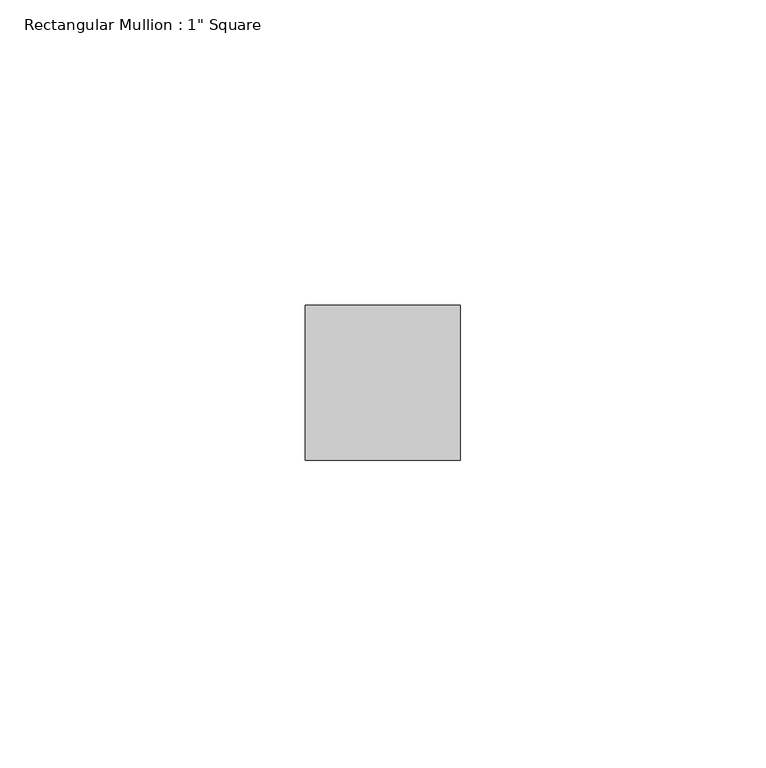
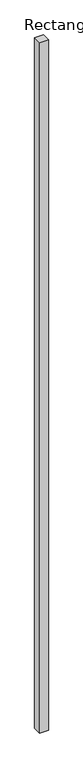
"""IFC4 building model written with IfcOpenShell, lengths in millimetres: member geometry."""

from ifc_helpers import new_model, si_unit, frame, origin, place, context, project, spatial, polyline, outline, extrude, source, transform, mapped, element, save


def member_8547658d(model_context):
    return source(origin(), model_context, "Body", "SweptSolid", [
        extrude(outline(polyline([(12.7, 12.7), (12.7, -12.7), (-12.7, -12.7), (-12.7, 12.7), (12.7, 12.7)])), frame((0.0, 0.0, -2146.3), z_axis=(0.0, 0.0, 1.0), x_axis=(1.0, 0.0, 0.0)), (0.0, 0.0, 1.0), 2146.3),
    ])


if __name__ == "__main__":
    model = new_model("IFC4")
    model_context = context("Model", 3, world=origin())
    ifc_project = project(units=[si_unit("LENGTHUNIT", "METRE", prefix="MILLI")], contexts=[model_context])
    site = spatial("IfcSite", under=ifc_project)
    building = spatial("IfcBuilding", under=site)
    placement = place(None, origin())
    member_shape = member_8547658d(model_context)
    element("IfcMember", 1, ObjectType="Rectangular Mullion : 1\" Square", at=placement, inside=building, context=model_context, shape_type="MappedRepresentation", body=[
        mapped(member_shape, transform((0.0, 0.0, 0.0), x_axis=(1.0, 0.0, 0.0), y_axis=(0.0, 1.0, 0.0), z_axis=(0.0, 0.0, 1.0))),
    ])
    save(model, "model.ifc")

# Revit data of these elements
# Type "Rectangular Mullion : 1\" Square"
#   built-in parameter 1007304 = 0.0833333 (stored number, unit not read)
#   built-in parameter 1007301 = 0.0416667 (stored number, unit not read)
#   built-in parameter 1007300 = 0.0416667 (stored number, unit not read)
# Element 1 (IfcMember, "Rectangular Mullion : 1\" Square")
#   Materials on its faces: "Aluminum"
# Materials
#   "Aluminum": class "Metal", colour RGB 247 247 247, transparency 0, Description = "Aluminum 6061", Cost = 0
